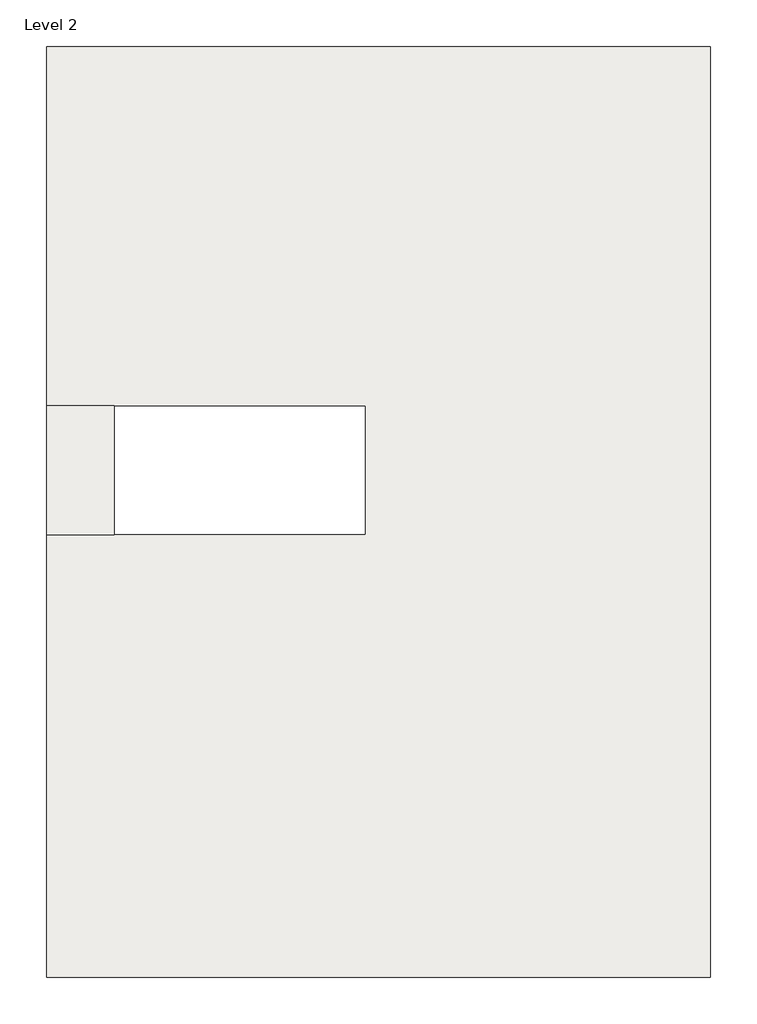
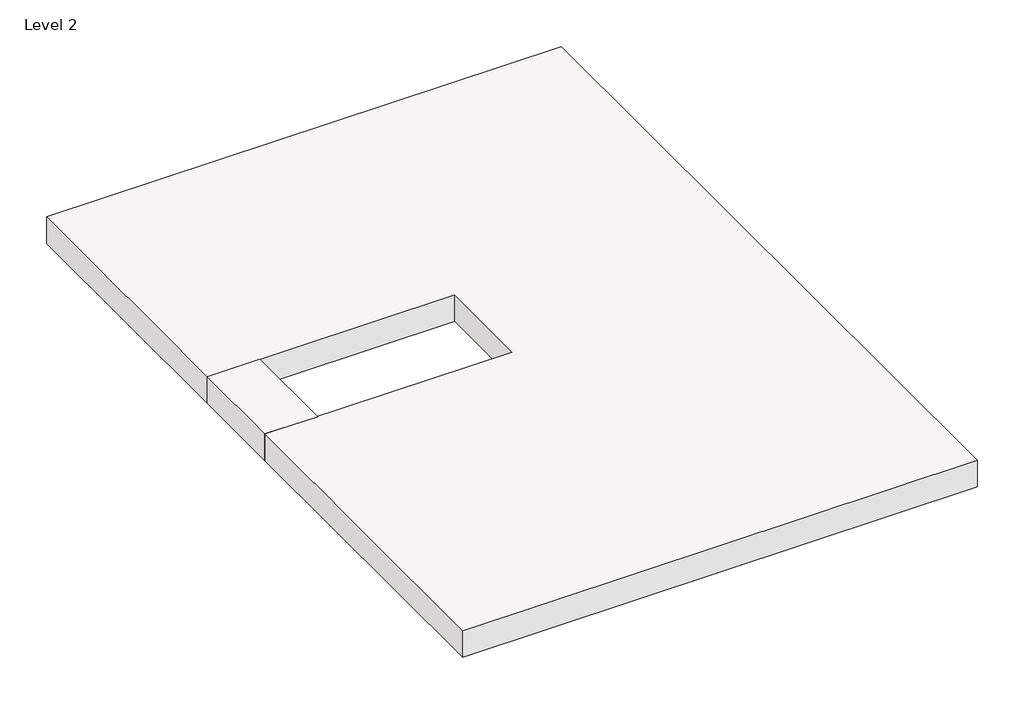
# One storey: 2 roofs.
"""IFC4 building model written with IfcOpenShell, lengths in millimetres."""

from ifc_helpers import new_model, si_unit, frame, origin, place, context, project, spatial, polyline, outline, extrude, element, save

model = new_model("IFC4")

# Units and contexts
model_context = context("Model", 3, world=origin())
ifc_project = project(units=[si_unit("LENGTHUNIT", "METRE", prefix="MILLI")], contexts=[model_context])

# Site, building, storey
site = spatial("IfcSite", under=ifc_project)
building = spatial("IfcBuilding", under=site)
storey = spatial("IfcBuildingStorey", under=building, Name="Level 2", Elevation=3048.0)

# Roofs
placement = place(None, origin())
element("IfcRoof", 1, ObjectType="Steel Truss - Insulation on Metal Deck - EPDM", at=placement, inside=storey, context=model_context, shape_type="SweptSolid", body=[
    extrude(outline(polyline([(-8480.28475, 12437.9839473), (1451.11525, 12437.9839473), (1451.11525, -1481.2160527), (-8480.28475, -1481.2160527), (-8480.28475, 5135.4839473), (-3705.08475, 5135.4839473), (-3705.08475, 7065.8839473), (-8480.28475, 7065.8839473), (-8480.28475, 12437.9839473)])), frame((0.0, 0.0, 3048.0), z_axis=(0.0, 0.0, 1.0), x_axis=(1.0, 0.0, 0.0)), (0.0, 0.0, 1.0), 546.1),
])
element("IfcRoof", 2, ObjectType="Steel Truss - Insulation on Metal Deck - EPDM", at=placement, inside=storey, context=model_context, shape_type="SweptSolid", body=[
    extrude(outline(polyline([(-8480.28475, 5135.4839473), (-8480.28475, 7065.8839473), (-7464.28475, 7065.8839473), (-7464.28475, 5135.4839473), (-8480.28475, 5135.4839473)])), frame((0.0, 0.0, 3048.0), z_axis=(0.0, 0.0, 1.0), x_axis=(1.0, 0.0, 0.0)), (0.0, 0.0, 1.0), 546.1),
])

save(model, "model.ifc")

# Revit data of these elements
# Type "Steel Truss - Insulation on Metal Deck - EPDM"
#   Assembly Code = "B1020"
#   Layers, outside or top first: 0' - 0 1/4" "Roofing, EPDM Membrane" (function 4); 0' - 5" "Rigid insulation" (function 3); 0' - 0 1/4" "Metal Deck" (function 1); 1' - 4" "Structure, Steel Bar Joist Layer" (function 1)
# Elements 1, 2 (IfcRoof, "Steel Truss - Insulation on Metal Deck - EPDM")
#   built-in parameter 1001705 = 11.7917 (stored number, unit not read)
#   built-in parameter 1001710 = 33615
#   Phase Created = New Construction
#   Materials on its faces: "Structure, Steel Bar Joist Layer", "Roofing, EPDM Membrane"
# Materials
#   "Roofing, EPDM Membrane": class "Generic", colour RGB 127 127 127, transparency 0, Description = "EPDM roof membrane", Cost = 0
#   "Rigid insulation": class "Generic", colour RGB 127 127 127, transparency 0, Description = "Rigid foam insulation board", Cost = 0
#   "Metal Deck": class "Metal", colour RGB 199 199 199, transparency 0, Description = "Steel, mill finish", Cost = 0
#   "Structure, Steel Bar Joist Layer": class "Metal", colour RGB 127 127 127, transparency 0, Description = "Bar joists, thermal airspace", Cost = 0
